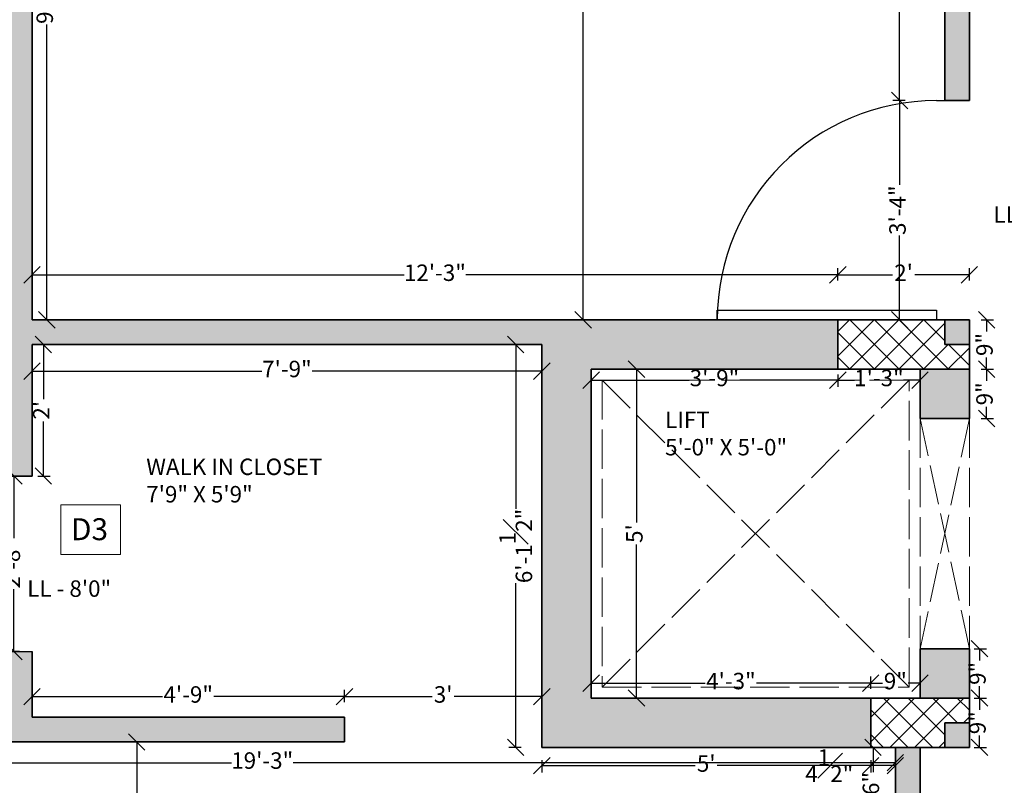
# Model space of a CAD drawing. Units: inches. Extents: x 1365 to 2091, y 1589 to 2091.
# Tile 3 of 8: x 1474 to 1654, y 1792 to 1932. Entities that reach past the tile are written whole.
import ezdxf

# ---------------------------------------------------------------- set-up
doc = ezdxf.new("R2010")
doc.units = ezdxf.units.IN
doc.linetypes.add('ACAD_ISO02W100', pattern=[15, 12, -3])
for name, color, linetype, lineweight in [('A-ANNO-DIMS', 2, 'Continuous', 18), ('A-ANNO-SYMB', 12, 'Continuous', 18), ('A-AREA-IDEN', 7, 'Continuous', 18), ('A-COLS', 7, 'Continuous', 35), ('A-COLS-MARK-PATT', 114, 'Continuous', 13), ('A-COLS-PATT', 1, 'Continuous', 13), ('A-DOOR', 4, 'Continuous', 25), ('A-EQPM-LIFT-HIDN', 254, 'ACAD_ISO02W100', 18), ('A-WALL', 7, 'Continuous', 35), ('A-WALL-PATT', 253, 'Continuous', 13)]:
    doc.layers.add(name, color=color, linetype=linetype, lineweight=lineweight)
doc.styles.get("Standard").update_dxf_attribs({"font": 'arial.ttf'})
doc.dimstyles.new('ISO-25', dxfattribs={"dimtxt": 3, "dimasz": 3, "dimexe": 1.25, "dimexo": 0.625, "dimtad": 0, "dimlunit": 4, "dimtxsty": 'Standard', "dimblk": 'OBLIQUE', "dimcen": 2.5, "dimclrd": 254, "dimclre": 254, "dimclrt": 1, "dimadec": 0, "dimazin": 0, "dimtfac": 1, "dimtmove": 0, "dimatfit": 3, "dimfxl": 1, "dimfxlon": 1, "dimfrac": 1, "dimarcsym": 0})

# ---------------------------------------------------------------- blocks, each defined once
blk = doc.blocks.new('*U4')
for p, q in [((0, 0), (0, -6)), ((32, 0), (32, -6))]:
    blk.add_line(p, q)
blk.add_lwpolyline([(0, 0), (0, 32), (1.75, 32), (1.75, 0)], close=True)
blk.add_arc((0, 0), 32, 0, 90)
blk = doc.blocks.new('*U5')
for p, q in [((0, 0), (0, -6)), ((40, 0), (40, -6))]:
    blk.add_line(p, q)
blk.add_lwpolyline([(0, 0), (0, 40), (1.75, 40), (1.75, 0)], close=True)
blk.add_arc((0, 0), 40, 0, 90)
blk = doc.blocks.new('_Oblique')
at = {"color": 0, "linetype": 'ByBlock', "lineweight": -2}
blk.add_line((-0.5, -0.5), (0.5, 0.5), dxfattribs=at)
blk = doc.blocks.new('*D34')
at = {"layer": 'A-ANNO-DIMS', "color": 0, "lineweight": -2, "transparency": 16777216}
for p, q in [((1473.96, 1848.36), (1471.71, 1848.36)), ((1472.96, 1848.36), (1472.96, 1837)), ((1472.96, 1816.36), (1472.96, 1827.72)), ((1473.96, 1816.36), (1471.71, 1816.36))]:
    blk.add_line(p, q, dxfattribs=at)
at = {"layer": 'Defpoints', "color": 0, "transparency": 16777216}
for p in [(1472.96, 1848.36), (1476.25, 1848.36), (1476.25, 1816.36)]:
    blk.add_point(p, dxfattribs=at)
at = {"layer": 'A-ANNO-DIMS', "color": 0, "lineweight": -2, "transparency": 16777216, "xscale": 3, "yscale": 3, "zscale": 3}
for p, rotation in [((1472.96, 1848.36), 90), ((1472.96, 1816.36), 270)]:
    blk.add_blockref('_Oblique', p, dxfattribs=dict(at, rotation=rotation))
at = {"layer": 'A-ANNO-DIMS', "color": 0, "transparency": 16777216, "insert": (1472.96, 1832.36), "char_height": 3, "attachment_point": 5, "rotation": 90}
blk.add_mtext('2\'-8"', dxfattribs=at)
blk = doc.blocks.new('*D35')
at = {"layer": 'A-ANNO-DIMS', "color": 0, "lineweight": -2, "transparency": 16777216}
for p, q in [((1477.32, 1872.36), (1479.57, 1872.36)), ((1478.32, 1872.36), (1478.32, 1862.39)), ((1478.32, 1848.36), (1478.32, 1858.33)), ((1477.32, 1848.36), (1479.57, 1848.36))]:
    blk.add_line(p, q, dxfattribs=at)
at = {"layer": 'Defpoints', "color": 0, "transparency": 16777216}
for p in [(1476.25, 1872.36), (1478.32, 1872.36), (1476.25, 1848.36)]:
    blk.add_point(p, dxfattribs=at)
at = {"layer": 'A-ANNO-DIMS', "color": 0, "lineweight": -2, "transparency": 16777216, "xscale": 3, "yscale": 3, "zscale": 3}
for p, rotation in [((1478.32, 1872.36), 90), ((1478.32, 1848.36), 270)]:
    blk.add_blockref('_Oblique', p, dxfattribs=dict(at, rotation=rotation))
at = {"layer": 'A-ANNO-DIMS', "color": 0, "transparency": 16777216, "insert": (1478.32, 1860.36), "char_height": 3, "attachment_point": 5, "rotation": 90}
blk.add_mtext("2'", dxfattribs=at)
blk = doc.blocks.new('*D36')
at = {"layer": 'A-ANNO-DIMS', "color": 0, "lineweight": -2, "transparency": 16777216}
for p, q in [((1476.25, 1807.13), (1476.25, 1809.38)), ((1533.25, 1807.13), (1533.25, 1809.38)), ((1476.25, 1808.13), (1500.08, 1808.13)), ((1533.25, 1808.13), (1509.43, 1808.13))]:
    blk.add_line(p, q, dxfattribs=at)
at = {"layer": 'Defpoints', "color": 0, "transparency": 16777216}
for p in [(1533.25, 1808.13), (1476.25, 1804.36), (1533.25, 1804.36)]:
    blk.add_point(p, dxfattribs=at)
at = {"layer": 'A-ANNO-DIMS', "color": 0, "lineweight": -2, "transparency": 16777216, "xscale": 3, "yscale": 3, "zscale": 3, "rotation": 180}
blk.add_blockref('_Oblique', (1476.25, 1808.13), dxfattribs=at)
at = {"layer": 'A-ANNO-DIMS', "color": 0, "lineweight": -2, "transparency": 16777216, "xscale": 3, "yscale": 3, "zscale": 3}
blk.add_blockref('_Oblique', (1533.25, 1808.13), dxfattribs=at)
at = {"layer": 'A-ANNO-DIMS', "color": 0, "transparency": 16777216, "insert": (1504.75, 1808.13), "char_height": 3, "attachment_point": 5}
blk.add_mtext('4\'-9"', dxfattribs=at)
blk = doc.blocks.new('*D37')
at = {"layer": 'A-ANNO-DIMS', "color": 0, "lineweight": -2, "transparency": 16777216}
for p, q in [((1533.25, 1807.13), (1533.25, 1809.38)), ((1569.25, 1808.13), (1569.25, 1809.38)), ((1533.25, 1808.13), (1549.25, 1808.13)), ((1569.25, 1808.13), (1553.26, 1808.13))]:
    blk.add_line(p, q, dxfattribs=at)
at = {"layer": 'Defpoints', "color": 0, "transparency": 16777216}
for p in [(1569.25, 1808.13), (1569.25, 1808.13), (1533.25, 1804.36)]:
    blk.add_point(p, dxfattribs=at)
at = {"layer": 'A-ANNO-DIMS', "color": 0, "lineweight": -2, "transparency": 16777216, "xscale": 3, "yscale": 3, "zscale": 3, "rotation": 180}
blk.add_blockref('_Oblique', (1533.25, 1808.13), dxfattribs=at)
at = {"layer": 'A-ANNO-DIMS', "color": 0, "lineweight": -2, "transparency": 16777216, "xscale": 3, "yscale": 3, "zscale": 3}
blk.add_blockref('_Oblique', (1569.25, 1808.13), dxfattribs=at)
at = {"layer": 'A-ANNO-DIMS', "color": 0, "transparency": 16777216, "insert": (1551.25, 1808.13), "char_height": 3, "attachment_point": 5}
blk.add_mtext("3'", dxfattribs=at)
blk = doc.blocks.new('*D38')
at = {"layer": 'A-ANNO-DIMS', "color": 0, "lineweight": -2, "transparency": 16777216}
for p, q in [((1565.49, 1872.36), (1563.24, 1872.36)), ((1564.49, 1872.36), (1564.49, 1842.37)), ((1564.49, 1798.86), (1564.49, 1828.84)), ((1565.49, 1798.86), (1563.24, 1798.86))]:
    blk.add_line(p, q, dxfattribs=at)
at = {"layer": 'Defpoints', "color": 0, "transparency": 16777216}
for p in [(1564.49, 1872.36), (1569.25, 1872.36), (1569.25, 1798.86)]:
    blk.add_point(p, dxfattribs=at)
at = {"layer": 'A-ANNO-DIMS', "color": 0, "lineweight": -2, "transparency": 16777216, "xscale": 3, "yscale": 3, "zscale": 3}
for p, rotation in [((1564.49, 1872.36), 90), ((1564.49, 1798.86), 270)]:
    blk.add_blockref('_Oblique', p, dxfattribs=dict(at, rotation=rotation))
at = {"layer": 'A-ANNO-DIMS', "color": 0, "transparency": 16777216, "insert": (1564.49, 1835.61), "char_height": 3, "attachment_point": 5, "rotation": 90}
blk.add_mtext('6\'-1{\\H1x;\\S1#2;}"', dxfattribs=at)
blk = doc.blocks.new('*D39')
at = {"layer": 'A-ANNO-DIMS', "color": 0, "lineweight": -2, "transparency": 16777216}
for p, q in [((1476.25, 1868.5), (1476.25, 1866.25)), ((1569.25, 1868.5), (1569.25, 1866.25)), ((1476.25, 1867.5), (1518.15, 1867.5)), ((1569.25, 1867.5), (1527.35, 1867.5))]:
    blk.add_line(p, q, dxfattribs=at)
at = {"layer": 'Defpoints', "color": 0, "transparency": 16777216}
for p in [(1476.25, 1872.36), (1569.25, 1872.36), (1569.25, 1867.5)]:
    blk.add_point(p, dxfattribs=at)
at = {"layer": 'A-ANNO-DIMS', "color": 0, "lineweight": -2, "transparency": 16777216, "xscale": 3, "yscale": 3, "zscale": 3, "rotation": 180}
blk.add_blockref('_Oblique', (1476.25, 1867.5), dxfattribs=at)
at = {"layer": 'A-ANNO-DIMS', "color": 0, "lineweight": -2, "transparency": 16777216, "xscale": 3, "yscale": 3, "zscale": 3}
blk.add_blockref('_Oblique', (1569.25, 1867.5), dxfattribs=at)
at = {"layer": 'A-ANNO-DIMS', "color": 0, "transparency": 16777216, "insert": (1522.75, 1867.5), "char_height": 3, "attachment_point": 5}
blk.add_mtext('7\'-9"', dxfattribs=at)
blk = doc.blocks.new('*D40')
at = {"layer": 'A-ANNO-DIMS', "color": 0, "lineweight": -2, "transparency": 16777216}
for p, q in [((1402.75, 1797.07), (1402.75, 1794.82)), ((1633.75, 1797.07), (1633.75, 1794.82)), ((1402.75, 1796.07), (1512.62, 1796.07)), ((1633.75, 1796.07), (1523.89, 1796.07))]:
    blk.add_line(p, q, dxfattribs=at)
at = {"layer": 'Defpoints', "color": 0, "transparency": 16777216}
for p in [(1402.75, 1799.86), (1633.75, 1798.86), (1633.75, 1796.07)]:
    blk.add_point(p, dxfattribs=at)
at = {"layer": 'A-ANNO-DIMS', "color": 0, "lineweight": -2, "transparency": 16777216, "xscale": 3, "yscale": 3, "zscale": 3, "rotation": 180}
blk.add_blockref('_Oblique', (1402.75, 1796.07), dxfattribs=at)
at = {"layer": 'A-ANNO-DIMS', "color": 0, "lineweight": -2, "transparency": 16777216, "xscale": 3, "yscale": 3, "zscale": 3}
blk.add_blockref('_Oblique', (1633.75, 1796.07), dxfattribs=at)
at = {"layer": 'A-ANNO-DIMS', "color": 0, "transparency": 16777216, "insert": (1518.25, 1796.07), "char_height": 3, "attachment_point": 5}
blk.add_mtext('19\'-3"', dxfattribs=at)
blk = doc.blocks.new('*D41')
at = {"layer": 'A-ANNO-DIMS', "color": 0, "lineweight": -2, "transparency": 16777216}
for p, q in [((1494.36, 1799.86), (1496.61, 1799.86)), ((1495.36, 1799.86), (1495.36, 1731.49)), ((1495.36, 1651.86), (1495.36, 1720.22)), ((1494.36, 1651.86), (1496.61, 1651.86))]:
    blk.add_line(p, q, dxfattribs=at)
at = {"layer": 'Defpoints', "color": 0, "transparency": 16777216}
for p in [(1482.35, 1799.86), (1482.35, 1651.86), (1495.36, 1651.86)]:
    blk.add_point(p, dxfattribs=at)
at = {"layer": 'A-ANNO-DIMS', "color": 0, "lineweight": -2, "transparency": 16777216, "xscale": 3, "yscale": 3, "zscale": 3}
for p, rotation in [((1495.36, 1799.86), 90), ((1495.36, 1651.86), 270)]:
    blk.add_blockref('_Oblique', p, dxfattribs=dict(at, rotation=rotation))
at = {"layer": 'A-ANNO-DIMS', "color": 0, "transparency": 16777216, "insert": (1495.36, 1725.86), "char_height": 3, "attachment_point": 5, "rotation": 90}
blk.add_mtext('12\'-4"', dxfattribs=at)
blk = doc.blocks.new('*D48')
at = {"layer": 'A-ANNO-DIMS', "color": 0, "lineweight": -2, "transparency": 16777216}
for p, q in [((1630.68, 1798.86), (1628.43, 1798.86)), ((1629.68, 1798.86), (1629.68, 1794.33)), ((1629.68, 1780.86), (1629.68, 1785.39)), ((1630.68, 1780.86), (1628.43, 1780.86))]:
    blk.add_line(p, q, dxfattribs=at)
at = {"layer": 'Defpoints', "color": 0, "transparency": 16777216}
for p in [(1633.75, 1798.86), (1629.68, 1780.86), (1633.75, 1780.86)]:
    blk.add_point(p, dxfattribs=at)
at = {"layer": 'A-ANNO-DIMS', "color": 0, "lineweight": -2, "transparency": 16777216, "xscale": 3, "yscale": 3, "zscale": 3}
for p, rotation in [((1629.68, 1798.86), 90), ((1629.68, 1780.86), 270)]:
    blk.add_blockref('_Oblique', p, dxfattribs=dict(at, rotation=rotation))
at = {"layer": 'A-ANNO-DIMS', "color": 0, "transparency": 16777216, "insert": (1629.68, 1789.86), "char_height": 3, "attachment_point": 5, "rotation": 90}
blk.add_mtext('1\'-6"', dxfattribs=at)
blk = doc.blocks.new('*D97')
at = {"layer": 'A-ANNO-DIMS', "color": 0, "lineweight": -2, "transparency": 16777216}
for p, q in [((1635.53, 1981.86), (1633.28, 1981.86)), ((1634.53, 1981.86), (1634.53, 1953.97)), ((1634.53, 1916.86), (1634.53, 1944.75)), ((1635.53, 1916.86), (1633.28, 1916.86))]:
    blk.add_line(p, q, dxfattribs=at)
at = {"layer": 'Defpoints', "color": 0, "transparency": 16777216}
for p in [(1642.75, 1981.86), (1634.53, 1916.86), (1642.75, 1916.86)]:
    blk.add_point(p, dxfattribs=at)
at = {"layer": 'A-ANNO-DIMS', "color": 0, "lineweight": -2, "transparency": 16777216, "xscale": 3, "yscale": 3, "zscale": 3}
for p, rotation in [((1634.53, 1981.86), 90), ((1634.53, 1916.86), 270)]:
    blk.add_blockref('_Oblique', p, dxfattribs=dict(at, rotation=rotation))
at = {"layer": 'A-ANNO-DIMS', "color": 0, "transparency": 16777216, "insert": (1634.53, 1949.36), "char_height": 3, "attachment_point": 5, "rotation": 90}
blk.add_mtext('5\'-5"', dxfattribs=at)
blk = doc.blocks.new('*D98')
at = {"layer": 'A-ANNO-DIMS', "color": 0, "lineweight": -2, "transparency": 16777216}
for p, q in [((1635.53, 1916.86), (1633.28, 1916.86)), ((1634.53, 1916.86), (1634.53, 1901.47)), ((1634.53, 1876.86), (1634.53, 1892.25)), ((1635.53, 1876.86), (1633.28, 1876.86))]:
    blk.add_line(p, q, dxfattribs=at)
at = {"layer": 'Defpoints', "color": 0, "transparency": 16777216}
for p in [(1642.75, 1916.86), (1634.53, 1876.86), (1647.25, 1876.86)]:
    blk.add_point(p, dxfattribs=at)
at = {"layer": 'A-ANNO-DIMS', "color": 0, "lineweight": -2, "transparency": 16777216, "xscale": 3, "yscale": 3, "zscale": 3}
for p, rotation in [((1634.53, 1916.86), 90), ((1634.53, 1876.86), 270)]:
    blk.add_blockref('_Oblique', p, dxfattribs=dict(at, rotation=rotation))
at = {"layer": 'A-ANNO-DIMS', "color": 0, "transparency": 16777216, "insert": (1634.53, 1896.86), "char_height": 3, "attachment_point": 5, "rotation": 90}
blk.add_mtext('3\'-4"', dxfattribs=at)
blk = doc.blocks.new('*D99')
at = {"layer": 'A-ANNO-DIMS', "color": 0, "lineweight": -2, "transparency": 16777216}
for p, q in [((1649.39, 1876.86), (1651.64, 1876.86)), ((1650.39, 1876.86), (1650.39, 1874.71)), ((1650.39, 1867.86), (1650.39, 1870.01)), ((1649.39, 1867.86), (1651.64, 1867.86))]:
    blk.add_line(p, q, dxfattribs=at)
at = {"layer": 'Defpoints', "color": 0, "transparency": 16777216}
for p in [(1647.25, 1876.86), (1647.25, 1867.86), (1650.39, 1867.86)]:
    blk.add_point(p, dxfattribs=at)
at = {"layer": 'A-ANNO-DIMS', "color": 0, "lineweight": -2, "transparency": 16777216, "xscale": 3, "yscale": 3, "zscale": 3}
for p, rotation in [((1650.39, 1876.86), 90), ((1650.39, 1867.86), 270)]:
    blk.add_blockref('_Oblique', p, dxfattribs=dict(at, rotation=rotation))
at = {"layer": 'A-ANNO-DIMS', "color": 0, "transparency": 16777216, "insert": (1650.39, 1872.36), "char_height": 3, "attachment_point": 5, "rotation": 90}
blk.add_mtext('9"', dxfattribs=at)
blk = doc.blocks.new('*D100')
at = {"layer": 'A-ANNO-DIMS', "color": 0, "lineweight": -2, "transparency": 16777216}
for p, q in [((1649.39, 1867.86), (1651.64, 1867.86)), ((1650.39, 1867.86), (1650.39, 1865.71)), ((1650.39, 1858.86), (1650.39, 1861.01)), ((1649.39, 1858.86), (1651.64, 1858.86))]:
    blk.add_line(p, q, dxfattribs=at)
at = {"layer": 'Defpoints', "color": 0, "transparency": 16777216}
for p in [(1647.25, 1867.86), (1647.25, 1858.86), (1650.39, 1858.86)]:
    blk.add_point(p, dxfattribs=at)
at = {"layer": 'A-ANNO-DIMS', "color": 0, "lineweight": -2, "transparency": 16777216, "xscale": 3, "yscale": 3, "zscale": 3}
for p, rotation in [((1650.39, 1867.86), 90), ((1650.39, 1858.86), 270)]:
    blk.add_blockref('_Oblique', p, dxfattribs=dict(at, rotation=rotation))
at = {"layer": 'A-ANNO-DIMS', "color": 0, "transparency": 16777216, "insert": (1650.39, 1863.36), "char_height": 3, "attachment_point": 5, "rotation": 90}
blk.add_mtext('9"', dxfattribs=at)
blk = doc.blocks.new('*D101')
at = {"layer": 'A-ANNO-DIMS', "color": 0, "lineweight": -2, "transparency": 16777216}
for p, q in [((1648.11, 1816.86), (1650.36, 1816.86)), ((1649.11, 1816.86), (1649.11, 1814.71)), ((1649.11, 1807.86), (1649.11, 1810.01)), ((1648.11, 1807.86), (1650.36, 1807.86))]:
    blk.add_line(p, q, dxfattribs=at)
at = {"layer": 'Defpoints', "color": 0, "transparency": 16777216}
for p in [(1647.25, 1816.86), (1647.25, 1807.86), (1649.11, 1807.86)]:
    blk.add_point(p, dxfattribs=at)
at = {"layer": 'A-ANNO-DIMS', "color": 0, "lineweight": -2, "transparency": 16777216, "xscale": 3, "yscale": 3, "zscale": 3}
for p, rotation in [((1649.11, 1816.86), 90), ((1649.11, 1807.86), 270)]:
    blk.add_blockref('_Oblique', p, dxfattribs=dict(at, rotation=rotation))
at = {"layer": 'A-ANNO-DIMS', "color": 0, "transparency": 16777216, "insert": (1649.11, 1812.36), "char_height": 3, "attachment_point": 5, "rotation": 90}
blk.add_mtext('9"', dxfattribs=at)
blk = doc.blocks.new('*D102')
at = {"layer": 'A-ANNO-DIMS', "color": 0, "lineweight": -2, "transparency": 16777216}
for p, q in [((1648.11, 1807.86), (1650.36, 1807.86)), ((1649.11, 1807.86), (1649.11, 1805.71)), ((1649.11, 1798.86), (1649.11, 1801.01)), ((1648.11, 1798.86), (1650.36, 1798.86))]:
    blk.add_line(p, q, dxfattribs=at)
at = {"layer": 'Defpoints', "color": 0, "transparency": 16777216}
for p in [(1647.25, 1807.86), (1647.25, 1798.86), (1649.11, 1798.86)]:
    blk.add_point(p, dxfattribs=at)
at = {"layer": 'A-ANNO-DIMS', "color": 0, "lineweight": -2, "transparency": 16777216, "xscale": 3, "yscale": 3, "zscale": 3}
for p, rotation in [((1649.11, 1807.86), 90), ((1649.11, 1798.86), 270)]:
    blk.add_blockref('_Oblique', p, dxfattribs=dict(at, rotation=rotation))
at = {"layer": 'A-ANNO-DIMS', "color": 0, "transparency": 16777216, "insert": (1649.11, 1803.36), "char_height": 3, "attachment_point": 5, "rotation": 90}
blk.add_mtext('9"', dxfattribs=at)
blk = doc.blocks.new('*D103')
at = {"layer": 'A-ANNO-DIMS', "color": 0, "lineweight": -2, "transparency": 16777216}
for p, q in [((1623.25, 1866.86), (1623.25, 1864.61)), ((1638.25, 1866.86), (1638.25, 1864.61)), ((1623.25, 1865.86), (1626.28, 1865.86)), ((1638.25, 1865.86), (1635.22, 1865.86))]:
    blk.add_line(p, q, dxfattribs=at)
at = {"layer": 'Defpoints', "color": 0, "transparency": 16777216}
for p in [(1623.25, 1867.86), (1638.25, 1867.86), (1623.25, 1865.86)]:
    blk.add_point(p, dxfattribs=at)
at = {"layer": 'A-ANNO-DIMS', "color": 0, "lineweight": -2, "transparency": 16777216, "xscale": 3, "yscale": 3, "zscale": 3, "rotation": 180}
blk.add_blockref('_Oblique', (1623.25, 1865.86), dxfattribs=at)
at = {"layer": 'A-ANNO-DIMS', "color": 0, "lineweight": -2, "transparency": 16777216, "xscale": 3, "yscale": 3, "zscale": 3}
blk.add_blockref('_Oblique', (1638.25, 1865.86), dxfattribs=at)
at = {"layer": 'A-ANNO-DIMS', "color": 0, "transparency": 16777216, "insert": (1630.75, 1865.86), "char_height": 3, "attachment_point": 5}
blk.add_mtext('1\'-3"', dxfattribs=at)
blk = doc.blocks.new('*D104')
at = {"layer": 'A-ANNO-DIMS', "color": 0, "lineweight": -2, "transparency": 16777216}
for p, q in [((1578.25, 1866.86), (1578.25, 1864.61)), ((1623.25, 1866.86), (1623.25, 1864.61)), ((1578.25, 1865.86), (1596.14, 1865.86)), ((1623.25, 1865.86), (1605.37, 1865.86))]:
    blk.add_line(p, q, dxfattribs=at)
at = {"layer": 'Defpoints', "color": 0, "transparency": 16777216}
for p in [(1578.25, 1867.86), (1623.25, 1867.86), (1578.25, 1865.86)]:
    blk.add_point(p, dxfattribs=at)
at = {"layer": 'A-ANNO-DIMS', "color": 0, "lineweight": -2, "transparency": 16777216, "xscale": 3, "yscale": 3, "zscale": 3, "rotation": 180}
blk.add_blockref('_Oblique', (1578.25, 1865.86), dxfattribs=at)
at = {"layer": 'A-ANNO-DIMS', "color": 0, "lineweight": -2, "transparency": 16777216, "xscale": 3, "yscale": 3, "zscale": 3}
blk.add_blockref('_Oblique', (1623.25, 1865.86), dxfattribs=at)
at = {"layer": 'A-ANNO-DIMS', "color": 0, "transparency": 16777216, "insert": (1600.75, 1865.86), "char_height": 3, "attachment_point": 5}
blk.add_mtext('3\'-9"', dxfattribs=at)
blk = doc.blocks.new('*D105')
at = {"layer": 'A-ANNO-DIMS', "color": 0, "lineweight": -2, "transparency": 16777216}
for p, q in [((1585.53, 1867.86), (1587.78, 1867.86)), ((1586.53, 1867.86), (1586.53, 1839.86)), ((1586.53, 1807.86), (1586.53, 1835.85)), ((1585.53, 1807.86), (1587.78, 1807.86))]:
    blk.add_line(p, q, dxfattribs=at)
at = {"layer": 'Defpoints', "color": 0, "transparency": 16777216}
for p in [(1578.25, 1867.86), (1578.25, 1807.86), (1586.53, 1807.86)]:
    blk.add_point(p, dxfattribs=at)
at = {"layer": 'A-ANNO-DIMS', "color": 0, "lineweight": -2, "transparency": 16777216, "xscale": 3, "yscale": 3, "zscale": 3}
for p, rotation in [((1586.53, 1867.86), 90), ((1586.53, 1807.86), 270)]:
    blk.add_blockref('_Oblique', p, dxfattribs=dict(at, rotation=rotation))
at = {"layer": 'A-ANNO-DIMS', "color": 0, "transparency": 16777216, "insert": (1586.53, 1837.86), "char_height": 3, "attachment_point": 5, "rotation": 90}
blk.add_mtext("5'", dxfattribs=at)
blk = doc.blocks.new('*D106')
at = {"layer": 'A-ANNO-DIMS', "color": 0, "lineweight": -2, "transparency": 16777216}
for p, q in [((1629.25, 1809.57), (1629.25, 1811.82)), ((1638.25, 1809.57), (1638.25, 1811.82)), ((1629.25, 1810.57), (1631.4, 1810.57)), ((1638.25, 1810.57), (1636.1, 1810.57))]:
    blk.add_line(p, q, dxfattribs=at)
at = {"layer": 'Defpoints', "color": 0, "transparency": 16777216}
for p in [(1629.25, 1810.57), (1629.25, 1807.86), (1638.25, 1807.86)]:
    blk.add_point(p, dxfattribs=at)
at = {"layer": 'A-ANNO-DIMS', "color": 0, "lineweight": -2, "transparency": 16777216, "xscale": 3, "yscale": 3, "zscale": 3, "rotation": 180}
blk.add_blockref('_Oblique', (1629.25, 1810.57), dxfattribs=at)
at = {"layer": 'A-ANNO-DIMS', "color": 0, "lineweight": -2, "transparency": 16777216, "xscale": 3, "yscale": 3, "zscale": 3}
blk.add_blockref('_Oblique', (1638.25, 1810.57), dxfattribs=at)
at = {"layer": 'A-ANNO-DIMS', "color": 0, "transparency": 16777216, "insert": (1633.75, 1810.57), "char_height": 3, "attachment_point": 5}
blk.add_mtext('9"', dxfattribs=at)
blk = doc.blocks.new('*D107')
at = {"layer": 'A-ANNO-DIMS', "color": 0, "lineweight": -2, "transparency": 16777216}
for p, q in [((1578.25, 1809.57), (1578.25, 1811.82)), ((1629.25, 1809.57), (1629.25, 1811.82)), ((1578.25, 1810.57), (1599.08, 1810.57)), ((1629.25, 1810.57), (1608.43, 1810.57))]:
    blk.add_line(p, q, dxfattribs=at)
at = {"layer": 'Defpoints', "color": 0, "transparency": 16777216}
for p in [(1578.25, 1810.57), (1578.25, 1807.86), (1629.25, 1807.86)]:
    blk.add_point(p, dxfattribs=at)
at = {"layer": 'A-ANNO-DIMS', "color": 0, "lineweight": -2, "transparency": 16777216, "xscale": 3, "yscale": 3, "zscale": 3, "rotation": 180}
blk.add_blockref('_Oblique', (1578.25, 1810.57), dxfattribs=at)
at = {"layer": 'A-ANNO-DIMS', "color": 0, "lineweight": -2, "transparency": 16777216, "xscale": 3, "yscale": 3, "zscale": 3}
blk.add_blockref('_Oblique', (1629.25, 1810.57), dxfattribs=at)
at = {"layer": 'A-ANNO-DIMS', "color": 0, "transparency": 16777216, "insert": (1603.75, 1810.57), "char_height": 3, "attachment_point": 5}
blk.add_mtext('4\'-3"', dxfattribs=at)
blk = doc.blocks.new('*D108')
at = {"layer": 'A-ANNO-DIMS', "color": 0, "lineweight": -2, "transparency": 16777216}
for p, q in [((1629.25, 1796.53), (1629.25, 1794.28)), ((1633.75, 1796.53), (1633.75, 1794.28)), ((1629.25, 1795.53), (1626.25, 1795.53)), ((1633.75, 1795.53), (1629.25, 1795.53))]:
    blk.add_line(p, q, dxfattribs=at)
at = {"layer": 'Defpoints', "color": 0, "transparency": 16777216}
for p in [(1629.25, 1798.86), (1633.75, 1798.86), (1629.25, 1795.53)]:
    blk.add_point(p, dxfattribs=at)
at = {"layer": 'A-ANNO-DIMS', "color": 0, "lineweight": -2, "transparency": 16777216, "xscale": 3, "yscale": 3, "zscale": 3, "rotation": 180}
blk.add_blockref('_Oblique', (1629.25, 1795.53), dxfattribs=at)
at = {"layer": 'A-ANNO-DIMS', "color": 0, "lineweight": -2, "transparency": 16777216, "xscale": 3, "yscale": 3, "zscale": 3}
blk.add_blockref('_Oblique', (1633.75, 1795.53), dxfattribs=at)
at = {"layer": 'A-ANNO-DIMS', "color": 0, "transparency": 16777216, "insert": (1621.7, 1795.53), "char_height": 3, "attachment_point": 5}
blk.add_mtext('4{\\H1x;\\S1#2;}"', dxfattribs=at)
blk = doc.blocks.new('*D109')
at = {"layer": 'A-ANNO-DIMS', "color": 0, "lineweight": -2, "transparency": 16777216}
for p, q in [((1569.25, 1796.53), (1569.25, 1794.28)), ((1629.25, 1796.53), (1629.25, 1794.28)), ((1569.25, 1795.53), (1597.25, 1795.53)), ((1629.25, 1795.53), (1601.26, 1795.53))]:
    blk.add_line(p, q, dxfattribs=at)
at = {"layer": 'Defpoints', "color": 0, "transparency": 16777216}
for p in [(1569.25, 1798.86), (1629.25, 1798.86), (1569.25, 1795.53)]:
    blk.add_point(p, dxfattribs=at)
at = {"layer": 'A-ANNO-DIMS', "color": 0, "lineweight": -2, "transparency": 16777216, "xscale": 3, "yscale": 3, "zscale": 3, "rotation": 180}
blk.add_blockref('_Oblique', (1569.25, 1795.53), dxfattribs=at)
at = {"layer": 'A-ANNO-DIMS', "color": 0, "lineweight": -2, "transparency": 16777216, "xscale": 3, "yscale": 3, "zscale": 3}
blk.add_blockref('_Oblique', (1629.25, 1795.53), dxfattribs=at)
at = {"layer": 'A-ANNO-DIMS', "color": 0, "transparency": 16777216, "insert": (1599.25, 1795.53), "char_height": 3, "attachment_point": 5}
blk.add_mtext("5'", dxfattribs=at)
blk = doc.blocks.new('*D112')
at = {"layer": 'A-ANNO-DIMS', "color": 0, "lineweight": -2, "transparency": 16777216}
for p, q in [((1477.96, 1993.86), (1480.21, 1993.86)), ((1478.96, 1993.86), (1478.96, 1939.97)), ((1478.96, 1876.86), (1478.96, 1930.75)), ((1477.96, 1876.86), (1480.21, 1876.86))]:
    blk.add_line(p, q, dxfattribs=at)
at = {"layer": 'Defpoints', "color": 0, "transparency": 16777216}
for p in [(1476.25, 1993.86), (1476.25, 1876.86), (1478.96, 1876.86)]:
    blk.add_point(p, dxfattribs=at)
at = {"layer": 'A-ANNO-DIMS', "color": 0, "lineweight": -2, "transparency": 16777216, "xscale": 3, "yscale": 3, "zscale": 3}
for p, rotation in [((1478.96, 1993.86), 90), ((1478.96, 1876.86), 270)]:
    blk.add_blockref('_Oblique', p, dxfattribs=dict(at, rotation=rotation))
at = {"layer": 'A-ANNO-DIMS', "color": 0, "transparency": 16777216, "insert": (1478.96, 1935.36), "char_height": 3, "attachment_point": 5, "rotation": 90}
blk.add_mtext('9\'-9"', dxfattribs=at)
blk = doc.blocks.new('*D113')
at = {"layer": 'A-ANNO-DIMS', "color": 0, "lineweight": -2, "transparency": 16777216}
for p, q in [((1476.25, 1884.06), (1476.25, 1886.31)), ((1623.25, 1884.06), (1623.25, 1886.31)), ((1476.25, 1885.06), (1544.12, 1885.06)), ((1623.25, 1885.06), (1555.39, 1885.06))]:
    blk.add_line(p, q, dxfattribs=at)
at = {"layer": 'Defpoints', "color": 0, "transparency": 16777216}
for p in [(1623.25, 1885.06), (1476.25, 1876.86), (1623.25, 1876.86)]:
    blk.add_point(p, dxfattribs=at)
at = {"layer": 'A-ANNO-DIMS', "color": 0, "lineweight": -2, "transparency": 16777216, "xscale": 3, "yscale": 3, "zscale": 3, "rotation": 180}
blk.add_blockref('_Oblique', (1476.25, 1885.06), dxfattribs=at)
at = {"layer": 'A-ANNO-DIMS', "color": 0, "lineweight": -2, "transparency": 16777216, "xscale": 3, "yscale": 3, "zscale": 3}
blk.add_blockref('_Oblique', (1623.25, 1885.06), dxfattribs=at)
at = {"layer": 'A-ANNO-DIMS', "color": 0, "transparency": 16777216, "insert": (1549.75, 1885.06), "char_height": 3, "attachment_point": 5}
blk.add_mtext('12\'-3"', dxfattribs=at)
blk = doc.blocks.new('*D114')
at = {"layer": 'A-ANNO-DIMS', "color": 0, "lineweight": -2, "transparency": 16777216}
for p, q in [((1623.25, 1884.06), (1623.25, 1886.31)), ((1647.25, 1884.06), (1647.25, 1886.31)), ((1623.25, 1885.06), (1633.22, 1885.06)), ((1647.25, 1885.06), (1637.28, 1885.06))]:
    blk.add_line(p, q, dxfattribs=at)
at = {"layer": 'Defpoints', "color": 0, "transparency": 16777216}
for p in [(1647.25, 1885.06), (1623.25, 1876.86), (1647.25, 1876.86)]:
    blk.add_point(p, dxfattribs=at)
at = {"layer": 'A-ANNO-DIMS', "color": 0, "lineweight": -2, "transparency": 16777216, "xscale": 3, "yscale": 3, "zscale": 3, "rotation": 180}
blk.add_blockref('_Oblique', (1623.25, 1885.06), dxfattribs=at)
at = {"layer": 'A-ANNO-DIMS', "color": 0, "lineweight": -2, "transparency": 16777216, "xscale": 3, "yscale": 3, "zscale": 3}
blk.add_blockref('_Oblique', (1647.25, 1885.06), dxfattribs=at)
at = {"layer": 'A-ANNO-DIMS', "color": 0, "transparency": 16777216, "insert": (1635.25, 1885.06), "char_height": 3, "attachment_point": 5}
blk.add_mtext("2'", dxfattribs=at)
blk = doc.blocks.new('*D116')
at = {"layer": 'A-ANNO-DIMS', "color": 0, "lineweight": -2, "transparency": 16777216}
for p, q in [((1575.79, 2053.86), (1578.04, 2053.86)), ((1576.79, 2053.86), (1576.79, 1970.99)), ((1576.79, 1876.86), (1576.79, 1959.72)), ((1575.79, 1876.86), (1578.04, 1876.86))]:
    blk.add_line(p, q, dxfattribs=at)
at = {"layer": 'Defpoints', "color": 0, "transparency": 16777216}
for p in [(1550.15, 2053.86), (1550.15, 1876.86), (1576.79, 1876.86)]:
    blk.add_point(p, dxfattribs=at)
at = {"layer": 'A-ANNO-DIMS', "color": 0, "lineweight": -2, "transparency": 16777216, "xscale": 3, "yscale": 3, "zscale": 3}
for p, rotation in [((1576.79, 2053.86), 90), ((1576.79, 1876.86), 270)]:
    blk.add_blockref('_Oblique', p, dxfattribs=dict(at, rotation=rotation))
at = {"layer": 'A-ANNO-DIMS', "color": 0, "transparency": 16777216, "insert": (1576.79, 1965.36), "char_height": 3, "attachment_point": 5, "rotation": 90}
blk.add_mtext('14\'-9"', dxfattribs=at)
blk = doc.blocks.new('OPENING-TAG-D1')
blk.add_lwpolyline([(6.13, 13.79), (17.02, 13.79), (17.02, 4.75), (6.13, 4.75)], close=True)
at = {"attachment_point": 1}
for s, width, insert, char_height in [('{D1}', 14.5136, (7.98, 11.34), 4), ('{LL - 8\'0"}', 24.3857, (0, 0), 3)]:
    blk.add_mtext_dynamic_manual_height_columns(s, width=width, gutter_width=12.5, heights=[0], dxfattribs=dict(at, insert=insert, char_height=char_height))

msp = doc.modelspace()

# ---------------------------------------------------------------- hatches: boundary and pattern name
at = {"layer": 'A-COLS-MARK-PATT'}
h = msp.add_hatch(color=256, dxfattribs=at)
h.dxf.hatch_style = 1
h.paths.add_polyline_path([(1398.254, 2062.858), (1393.754, 2062.858), (1393.754, 2058.358), (1398.254, 2058.358)])
h.paths.add_polyline_path([(1398.254, 1872.358), (1393.754, 1872.358), (1393.754, 1867.858), (1398.254, 1867.858)])
h.paths.add_polyline_path([(1398.254, 1807.858), (1393.754, 1807.858), (1393.754, 1803.358), (1398.254, 1803.358)])
h.paths.add_polyline_path([(1398.254, 1647.358), (1393.754, 1647.358), (1393.754, 1642.858), (1398.254, 1642.858)])
h.paths.add_polyline_path([(1638.254, 1647.358), (1633.754, 1647.358), (1633.754, 1642.858), (1638.254, 1642.858)])
h.paths.add_polyline_path([(1638.254, 1732.858), (1633.754, 1732.858), (1633.754, 1728.358), (1638.254, 1728.358)])
h.paths.add_polyline_path([(1647.254, 1876.858), (1642.754, 1876.858), (1642.754, 1872.358), (1647.254, 1872.358)])
h.paths.add_polyline_path([(1647.254, 1803.358), (1642.754, 1803.358), (1642.754, 1798.858), (1647.254, 1798.858)])
h.paths.add_polyline_path([(1647.254, 2062.858), (1642.754, 2062.858), (1642.754, 2058.358), (1647.254, 2058.358)])
h.paths.add_polyline_path([(1824.254, 2062.858), (1819.754, 2062.858), (1819.754, 2058.358), (1824.254, 2058.358)])
h.paths.add_polyline_path([(1824.254, 1885.858), (1819.754, 1885.858), (1819.754, 1881.358), (1824.254, 1881.358)])
h.paths.add_polyline_path([(1828.754, 1647.358), (1824.254, 1647.358), (1824.254, 1642.858), (1828.754, 1642.858)])
h.paths.add_polyline_path([(1948.754, 1647.358), (1944.254, 1647.358), (1944.254, 1642.858), (1948.754, 1642.858)])
h.paths.add_polyline_path([(2041.754, 1647.358), (2037.254, 1647.358), (2037.254, 1642.858), (2041.754, 1642.858)])
h.paths.add_polyline_path([(2041.754, 1885.858), (2037.254, 1885.858), (2037.254, 1881.358), (2041.754, 1881.358)])
h.paths.add_polyline_path([(2041.754, 2062.858), (2037.254, 2062.858), (2037.254, 2058.358), (2041.754, 2058.358)])
at = {"layer": 'A-COLS-PATT'}
h = msp.add_hatch(dxfattribs=at)
h.set_pattern_fill('ANSI37', color=256)
h.paths.add_polyline_path([(1642.754, 1803.358), (1647.254, 1803.358), (1647.254, 1807.858), (1629.254, 1807.858), (1629.254, 1798.858), (1633.754, 1798.858), (1642.754, 1798.858)])
h.paths.add_polyline_path([(1647.254, 1872.358), (1642.754, 1872.358), (1642.754, 1876.858), (1641.254, 1876.858), (1623.254, 1876.858), (1623.254, 1867.858), (1638.254, 1867.858), (1647.254, 1867.858)])
h.paths.add_polyline_path([(1647.254, 2058.358), (1642.754, 2058.358), (1642.754, 2062.858), (1638.254, 2062.858), (1638.254, 2053.858), (1647.254, 2053.858)])
h.paths.add_polyline_path([(1642.754, 2053.858), (1638.254, 2053.858), (1638.254, 2041.858), (1642.754, 2041.858)])
h.paths.add_polyline_path([(1647.254, 2053.858), (1642.754, 2053.858), (1642.754, 2041.858), (1647.254, 2041.858)])
h.paths.add_polyline_path([(1828.754, 2062.858), (1824.254, 2062.858), (1824.254, 2058.358), (1819.754, 2058.358), (1819.754, 2038.858), (1828.754, 2038.858)])
h.paths.add_polyline_path([(1839.254, 1885.858), (1825.754, 1885.858), (1824.254, 1885.858), (1824.254, 1881.358), (1819.754, 1881.358), (1819.754, 1876.858), (1839.254, 1876.858)])
h.paths.add_polyline_path([(2041.754, 1881.358), (2037.254, 1881.358), (2037.254, 1885.858), (2023.754, 1885.858), (2023.754, 1876.858), (2041.754, 1876.858)])
h.paths.add_polyline_path([(1828.754, 1666.858), (1819.754, 1666.858), (1819.754, 1642.858), (1824.254, 1642.858), (1824.254, 1647.358), (1828.754, 1647.358)])
h.paths.add_polyline_path([(1944.254, 1647.358), (1948.754, 1647.358), (1948.754, 1651.858), (1930.754, 1651.858), (1930.754, 1642.858), (1944.254, 1642.858)])
h.paths.add_polyline_path([(2037.254, 1647.358), (2041.754, 1647.358), (2041.754, 1651.858), (2023.754, 1651.858), (2023.754, 1642.858), (2037.254, 1642.858)])
at = {"layer": 'A-WALL-PATT'}
h = msp.add_hatch(color=256, dxfattribs=at)
h.dxf.hatch_style = 1
h.paths.add_polyline_path([(1638.254, 2053.858), (1638.254, 2062.858), (1617.254, 2062.858), (1617.254, 2053.858)])
h.paths.add_polyline_path([(1633.754, 1780.858), (1638.254, 1780.858), (1638.254, 1798.858), (1633.754, 1798.858)])
h.paths.add_polyline_path([(1828.754, 2038.858), (1819.754, 2038.858), (1819.754, 1925.829), (1828.754, 1925.829)])
h = msp.add_hatch(color=256, dxfattribs=at)
h.dxf.hatch_style = 1
h.paths.add_polyline_path([(1402.754, 2053.858), (1393.754, 2053.858), (1393.754, 2029.858), (1402.754, 2029.858)])
h.paths.add_polyline_path([(1402.754, 2005.858), (1393.754, 2005.858), (1393.754, 1888.858), (1402.754, 1888.858)])
h.paths.add_polyline_path([(1444.754, 1984.858), (1402.754, 1984.858), (1402.754, 1975.858), (1444.754, 1975.858)], flags=17)
h.paths.add_polyline_path([(1476.254, 1993.858), (1471.754, 1993.858), (1471.754, 1933.858), (1402.754, 1933.858), (1402.754, 1929.358), (1471.754, 1929.358), (1471.754, 1848.358), (1476.254, 1848.358), (1476.254, 1872.358), (1569.254, 1872.358), (1569.254, 1798.858), (1573.754, 1798.858), (1629.254, 1798.858), (1629.254, 1807.858), (1578.254, 1807.858), (1578.254, 1867.858), (1623.254, 1867.858), (1623.254, 1876.858), (1476.254, 1876.858)])
h.paths.add_polyline_path([(1402.754, 1867.858), (1393.754, 1867.858), (1393.754, 1849.858), (1402.754, 1849.858)])
h.paths.add_polyline_path([(1402.754, 1825.858), (1393.754, 1825.858), (1393.754, 1807.858), (1398.254, 1807.858), (1402.754, 1807.858)])
h = msp.add_hatch(color=256, dxfattribs=at)
h.dxf.hatch_style = 1
h.paths.add_polyline_path([(1647.254, 2041.858), (1642.754, 2041.858), (1642.754, 2029.858), (1647.254, 2029.858)])
h.paths.add_polyline_path([(1647.254, 1981.858), (1642.754, 1981.858), (1642.754, 1916.858), (1647.254, 1916.858)])
h = msp.add_hatch(color=256, dxfattribs=at)
h.dxf.hatch_style = 1
h.paths.add_polyline_path([(1647.254, 1867.858), (1638.254, 1867.858), (1638.254, 1858.858), (1647.254, 1858.858)])
h = msp.add_hatch(color=256, dxfattribs=at)
h.dxf.hatch_style = 1
h.paths.add_polyline_path([(1402.754, 1753.858), (1393.754, 1753.858), (1393.754, 1663.858), (1402.754, 1663.858)])
h.paths.add_polyline_path([(1533.254, 1804.358), (1476.254, 1804.358), (1476.254, 1816.358), (1471.754, 1816.358), (1471.754, 1804.358), (1402.754, 1804.358), (1402.754, 1799.858), (1533.254, 1799.858)])
h.paths.add_polyline_path([(1638.254, 1714.858), (1633.754, 1714.858), (1633.754, 1666.858), (1638.254, 1666.858)])
h.paths.add_polyline_path([(1638.254, 1740.858), (1633.754, 1740.858), (1633.754, 1732.858), (1638.254, 1732.858)])
h.paths.add_polyline_path([(1954.754, 1744.858), (1948.754, 1744.858), (1944.254, 1744.858), (1824.254, 1744.858), (1824.254, 1821.858), (1819.754, 1821.858), (1819.754, 1666.858), (1824.254, 1666.858), (1824.254, 1740.358), (1944.254, 1740.358), (1948.754, 1740.358), (1954.754, 1740.358)])
h.paths.add_polyline_path([(1948.754, 1698.358), (1944.254, 1698.358), (1944.254, 1651.858), (1948.754, 1651.858)])
h.paths.add_polyline_path([(1948.754, 1740.358), (1944.254, 1740.358), (1944.254, 1734.358), (1948.754, 1734.358)], flags=17)
h = msp.add_hatch(color=256, dxfattribs=at)
h.dxf.hatch_style = 1
h.paths.add_polyline_path([(1647.254, 1816.858), (1638.254, 1816.858), (1638.254, 1807.858), (1647.254, 1807.858)])

# ---------------------------------------------------------------- linework, layer by layer
at = {"layer": 'A-ANNO-SYMB'}
msp.add_lwpolyline([(1481.507, 1843.113), (1492.396, 1843.113), (1492.396, 1834.075), (1481.507, 1834.075)], close=True, dxfattribs=at)
at = {"layer": 'A-COLS'}
for p, q in [((1623.254, 1867.858), (1623.254, 1876.858)), ((1642.754, 1872.358), (1642.754, 1876.858)), ((1647.254, 1876.858), (1647.254, 1872.358)), ((1647.254, 1872.358), (1642.754, 1872.358)), ((1638.254, 1867.858), (1623.254, 1867.858)), ((1629.254, 1798.858), (1629.254, 1807.858)), ((1629.254, 1807.858), (1629.254, 1807.858)), ((1647.254, 1803.358), (1642.754, 1803.358)), ((1642.754, 1803.358), (1642.754, 1798.858)), ((1647.254, 1798.858), (1647.254, 1803.358)), ((1633.754, 1798.858), (1629.254, 1798.858))]:
    msp.add_line(p, q, dxfattribs=at)
at = {"layer": 'A-EQPM-LIFT-HIDN', "ltscale": 0.6}
for p, q in [((1636.254, 1865.858), (1580.254, 1865.858)), ((1580.254, 1865.858), (1580.254, 1809.858)), ((1580.254, 1865.858), (1636.254, 1809.858)), ((1580.254, 1809.858), (1636.254, 1865.858)), ((1636.254, 1809.858), (1636.254, 1865.858)), ((1638.254, 1858.858), (1638.254, 1816.858)), ((1647.254, 1816.858), (1638.254, 1858.858)), ((1647.254, 1858.858), (1638.254, 1816.858)), ((1647.254, 1858.858), (1647.254, 1816.858)), ((1580.254, 1809.858), (1636.254, 1809.858))]:
    msp.add_line(p, q, dxfattribs=at)
at = {"layer": 'A-WALL'}
for p, q in [((1647.254, 1916.858), (1647.254, 2062.858)), ((1476.254, 1993.858), (1476.254, 1876.858)), ((1642.754, 1981.858), (1642.754, 1916.858)), ((1642.754, 1916.858), (1647.254, 1916.858)), ((1476.254, 1876.858), (1647.254, 1876.858)), ((1647.254, 1876.858), (1647.254, 1858.858)), ((1569.254, 1872.358), (1476.254, 1872.358)), ((1476.254, 1848.358), (1476.254, 1872.358)), ((1569.254, 1798.858), (1569.254, 1872.358)), ((1647.254, 1867.858), (1578.254, 1867.858)), ((1578.254, 1867.858), (1578.254, 1807.858)), ((1638.254, 1858.858), (1638.254, 1867.858)), ((1647.254, 1858.858), (1638.254, 1858.858)), ((1471.754, 1848.358), (1476.254, 1848.358)), ((1476.254, 1816.358), (1476.254, 1804.358)), ((1638.254, 1807.858), (1638.254, 1816.858)), ((1638.254, 1816.858), (1647.254, 1816.858)), ((1647.254, 1816.858), (1647.254, 1798.858)), ((1578.254, 1807.858), (1647.254, 1807.858)), ((1476.254, 1804.358), (1533.254, 1804.358)), ((1533.254, 1804.358), (1533.254, 1799.858)), ((1533.254, 1799.858), (1402.754, 1799.858)), ((1573.754, 1798.858), (1569.254, 1798.858)), ((1633.754, 1798.858), (1573.754, 1798.858)), ((1647.254, 1798.858), (1633.754, 1798.858)), ((1633.754, 1780.858), (1633.754, 1798.858)), ((1638.254, 1798.858), (1638.254, 1780.858))]:
    msp.add_line(p, q, dxfattribs=at)

# ---------------------------------------------------------------- block references
at = {"layer": 'A-ANNO-SYMB'}
msp.add_blockref('OPENING-TAG-D1', (1651.651, 1897.551), dxfattribs=at)
at = {"layer": 'A-DOOR'}
for name, p, rotation in [('*U5', (1641.254, 1876.858), 90), ('*U4', (1470.254, 1816.358), 89.99999999999999)]:
    msp.add_blockref(name, p, dxfattribs=dict(at, rotation=rotation))

# ---------------------------------------------------------------- texts
at = {"layer": 'A-ANNO-SYMB', "attachment_point": 1}
for s, width, insert, char_height in [('{D3}', 14.51356, (1483.347, 1840.662), 4), ('{LL - 8\'0"}', 24.3857, (1475.372, 1829.327), 3)]:
    msp.add_mtext_dynamic_manual_height_columns(s, width=width, gutter_width=12.5, heights=[0], dxfattribs=dict(at, insert=insert, char_height=char_height))
at = {"layer": 'A-AREA-IDEN', "char_height": 3, "attachment_point": 1}
for s, width, insert in [('{LIFT\\P5\'-0" X 5\'-0"}', 32.41055, (1591.742, 1860.127)), ('{WALK IN CLOSET\\P7\'9" X 5\'9"}', 40.48762, (1497.089, 1851.545))]:
    msp.add_mtext_dynamic_manual_height_columns(s, width=width, gutter_width=12.5, heights=[0], dxfattribs=dict(at, insert=insert))

# ---------------------------------------------------------------- dimensions: what is measured, and where the dimension line sits
at = {"layer": 'A-ANNO-DIMS'}
for base, p1, p2, override, picture, middle in [((1576.793, 1876.858), (1550.148, 2053.858), (1550.148, 1876.858), {"dimclrd": 0, "dimclre": 0, "dimclrt": 0}, '*D116', (1576.793, 1965.358)), ((1478.964, 1876.858), (1476.254, 1993.858), (1476.254, 1876.858), {"dimclrd": 0, "dimclre": 0, "dimclrt": 0, "dimtmove": 1}, '*D112', (1478.964, 1935.358)), ((1634.534, 1916.858), (1642.754, 1981.858), (1642.754, 1916.858), {"dimclrd": 0, "dimclre": 0, "dimclrt": 0, "dimtmove": 1}, '*D97', (1634.534, 1949.358)), ((1634.534, 1876.858), (1642.754, 1916.858), (1647.254, 1876.858), {"dimclrd": 0, "dimclre": 0, "dimclrt": 0, "dimtmove": 1}, '*D98', (1634.534, 1896.858)), ((1650.394, 1867.858), (1647.254, 1876.858), (1647.254, 1867.858), {"dimclrd": 0, "dimclre": 0, "dimclrt": 0}, '*D99', (1650.394, 1872.358)), ((1478.324, 1872.358), (1476.254, 1848.358), (1476.254, 1872.358), {"dimclrd": 0, "dimclre": 0, "dimclrt": 0}, '*D35', (1478.324, 1860.358)), ((1564.485, 1872.358), (1569.254, 1798.858), (1569.254, 1872.358), {"dimclrd": 0, "dimclre": 0, "dimclrt": 0}, '*D38', (1564.485, 1835.608)), ((1586.532, 1807.858), (1578.254, 1867.858), (1578.254, 1807.858), {"dimclrd": 0, "dimclre": 0, "dimclrt": 0}, '*D105', (1586.532, 1837.858)), ((1650.394, 1858.858), (1647.254, 1867.858), (1647.254, 1858.858), {"dimclrd": 0, "dimclre": 0, "dimclrt": 0, "dimtmove": 1}, '*D100', (1650.394, 1863.358)), ((1472.962, 1848.358), (1476.254, 1816.358), (1476.254, 1848.358), {"dimclrd": 0, "dimclre": 0, "dimclrt": 0}, '*D34', (1472.962, 1832.358)), ((1649.114, 1807.858), (1647.254, 1816.858), (1647.254, 1807.858), {"dimclrd": 0, "dimclre": 0, "dimclrt": 0}, '*D101', (1649.114, 1812.358)), ((1649.114, 1798.858), (1647.254, 1807.858), (1647.254, 1798.858), {"dimclrd": 0, "dimclre": 0, "dimclrt": 0, "dimtmove": 1}, '*D102', (1649.114, 1803.358)), ((1495.361, 1651.858), (1482.353, 1799.858), (1482.353, 1651.858), {"dimclrd": 0, "dimclre": 0, "dimclrt": 0}, '*D41', (1495.361, 1725.858)), ((1629.681, 1780.858), (1633.754, 1798.858), (1633.754, 1780.858), {"dimclrd": 0, "dimclre": 0, "dimclrt": 0}, '*D48', (1629.681, 1789.858))]:
    dim = msp.add_linear_dim(base=base, p1=p1, p2=p2, angle=90, dimstyle='ISO-25', override=override, dxfattribs=at)
    dim.commit()
    dim.dimension.update_dxf_attribs({"geometry": picture, "text_midpoint": middle})
for base, p1, p2, override, picture, middle in [((1623.254, 1885.059), (1476.254, 1876.858), (1623.254, 1876.858), {"dimclrd": 0, "dimclre": 0, "dimclrt": 0}, '*D113', (1549.754, 1885.059)), ((1647.254, 1885.059), (1623.254, 1876.858), (1647.254, 1876.858), {"dimclrd": 0, "dimclre": 0, "dimclrt": 0, "dimtmove": 1}, '*D114', (1635.254, 1885.059)), ((1569.254, 1867.505), (1476.254, 1872.358), (1569.254, 1872.358), {"dimclrd": 0, "dimclre": 0, "dimclrt": 0}, '*D39', (1522.754, 1867.505)), ((1578.254, 1865.858), (1623.254, 1867.858), (1578.254, 1867.858), {"dimclrd": 0, "dimclre": 0, "dimclrt": 0, "dimtmove": 1}, '*D104', (1600.754, 1865.858)), ((1623.254, 1865.858), (1638.254, 1867.858), (1623.254, 1867.858), {"dimclrd": 0, "dimclre": 0, "dimclrt": 0}, '*D103', (1630.754, 1865.858)), ((1578.254, 1810.574), (1629.254, 1807.858), (1578.254, 1807.858), {"dimclrd": 0, "dimclre": 0, "dimclrt": 0, "dimtmove": 1}, '*D107', (1603.754, 1810.574)), ((1629.254, 1810.574), (1638.254, 1807.858), (1629.254, 1807.858), {"dimclrd": 0, "dimclre": 0, "dimclrt": 0}, '*D106', (1633.754, 1810.574)), ((1533.254, 1808.13), (1476.254, 1804.358), (1533.254, 1804.358), {"dimclrd": 0, "dimclre": 0, "dimclrt": 0}, '*D36', (1504.754, 1808.13)), ((1569.254, 1808.13), (1533.254, 1804.358), (1569.254, 1808.13), {"dimclrd": 0, "dimclre": 0, "dimclrt": 0, "dimtmove": 1}, '*D37', (1551.254, 1808.13)), ((1633.754, 1796.07), (1402.754, 1799.858), (1633.754, 1798.858), {"dimclrd": 0, "dimclre": 0, "dimclrt": 0}, '*D40', (1518.254, 1796.07)), ((1569.254, 1795.532), (1629.254, 1798.858), (1569.254, 1798.858), {"dimclrd": 0, "dimclre": 0, "dimclrt": 0, "dimtmove": 1}, '*D109', (1599.254, 1795.532)), ((1629.254, 1795.532), (1633.754, 1798.858), (1629.254, 1798.858), {"dimclrd": 0, "dimclre": 0, "dimclrt": 0}, '*D108', (1621.698, 1795.532))]:
    dim = msp.add_linear_dim(base=base, p1=p1, p2=p2, dimstyle='ISO-25', override=override, dxfattribs=at)
    dim.commit()
    dim.dimension.update_dxf_attribs({"geometry": picture, "text_midpoint": middle})

doc.saveas('drawing.dxf')
